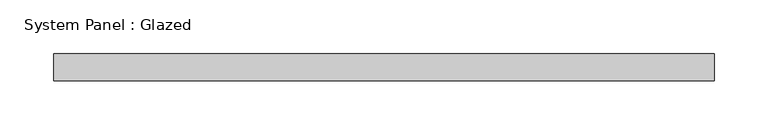
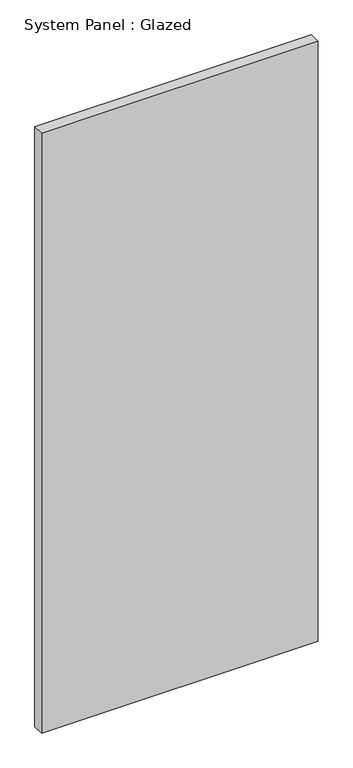
"""IFC4 building model written with IfcOpenShell, lengths in millimetres: plate geometry, System Panel : Glazed."""

from ifc_helpers import new_model, si_unit, origin, origin_with_axes, place, context, project, spatial, polyline, outline, extrude, source, transform, mapped, element, save


def system_panel_glazed_bbfcf774(model_context):
    return source(origin(), model_context, "Body", "SweptSolid", [
        extrude(outline(polyline([(307.975, 19.05), (-307.975, 19.05), (-307.975, 44.45), (307.975, 44.45), (307.975, 19.05)])), origin_with_axes(), (0.0, 0.0, 1.0), 1411.1940157),
    ])


if __name__ == "__main__":
    model = new_model("IFC4")
    model_context = context("Model", 3, world=origin())
    ifc_project = project(units=[si_unit("LENGTHUNIT", "METRE", prefix="MILLI")], contexts=[model_context])
    site = spatial("IfcSite", under=ifc_project)
    building = spatial("IfcBuilding", under=site)
    placement = place(None, origin())
    system_panel_glazed_shape = system_panel_glazed_bbfcf774(model_context)
    element("IfcPlate", 1, ObjectType="System Panel : Glazed", at=placement, inside=building, context=model_context, shape_type="MappedRepresentation", body=[
        mapped(system_panel_glazed_shape, transform((0.0, 0.0, 0.0), x_axis=(1.0, 0.0, 0.0), y_axis=(0.0, 1.0, 0.0), z_axis=(0.0, 0.0, 1.0))),
    ])
    save(model, "model.ifc")

# Revit data of these elements
# Type "System Panel : Glazed"
#   Construction Type Id = "GSP4R"
#   Analytic Construction = "1/8 in Pilkington single glazing"
#   Visual Light Transmittance = 0.9
#   Solar Heat Gain Coefficient = 0.86
#   Heat Transfer Coefficient (U) = 1.18115 BTU/(h·ft²·°F)
#   Define Thermal Properties by = 1
# Element 1 (IfcPlate, "System Panel : Glazed")
#   Materials on its faces: "Glass"
# Materials
#   "Glass": class "Glass", colour RGB 0 128 192, transparency 0.75, Description = "Soda Lime Glass", Cost = 0
